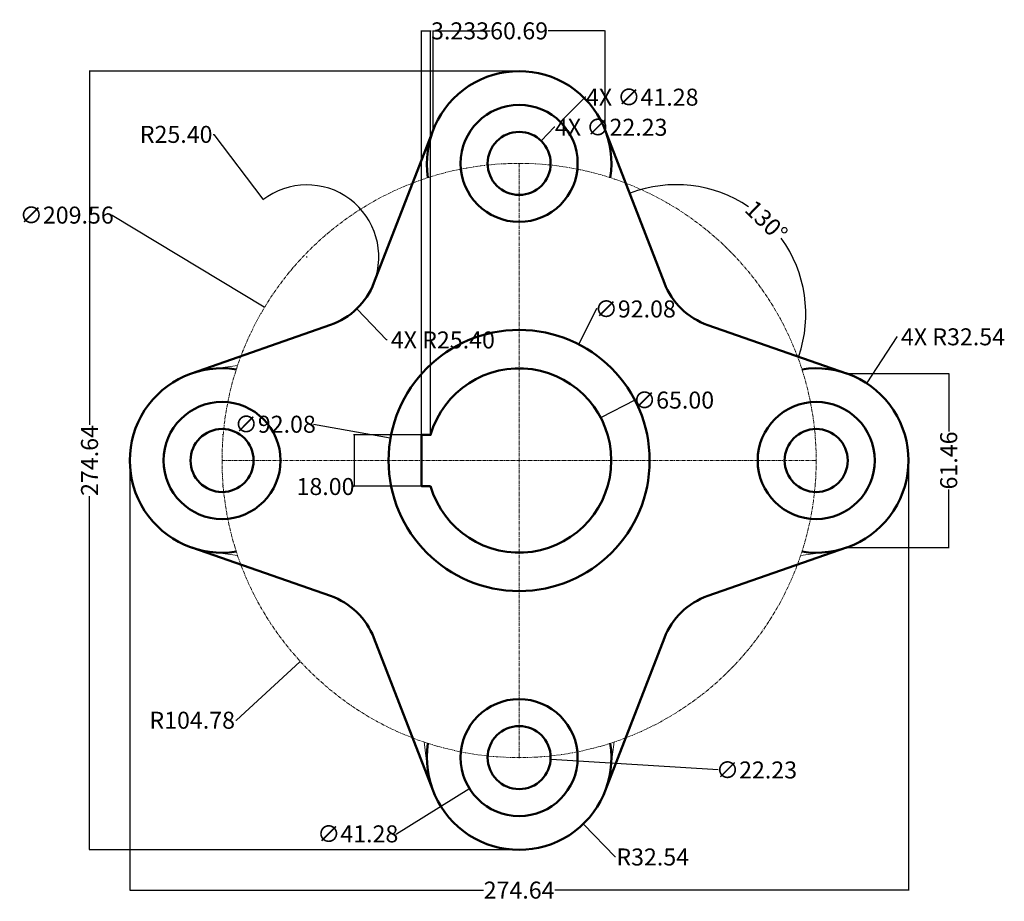
# Model space of a CAD drawing. Units: millimetres. Extents: x 95 to 442, y 57 to 368.
import ezdxf

# ---------------------------------------------------------------- set-up
doc = ezdxf.new("R2010")
doc.units = ezdxf.units.MM
doc.header["$MEASUREMENT"] = 0
doc.linetypes.add('CENTER', pattern=[2, 1.25, -0.25, 0.25, -0.25])
for name, color, linetype, lineweight in [('M-CNTR', 4, 'CENTER', 18), ('M-CONS', 8, 'Continuous', 13), ('M-DIMS', 2, 'Continuous', 25), ('M-OUTL', 7, 'Continuous', 50)]:
    doc.layers.add(name, color=color, linetype=linetype, lineweight=lineweight)
doc.styles.get("Standard").update_dxf_attribs({"font": 'arial.ttf'})
doc.dimstyles.get("Standard").update_dxf_attribs({"dimtxt": 6, "dimasz": 0.18, "dimexe": 0.18, "dimexo": 0.0625, "dimgap": 0.09, "dimtad": 0, "dimtoh": 1, "dimzin": 0, "dimdsep": 46, "dimtxsty": 'Standard', "dimcen": 0.09, "dimadec": 0, "dimazin": 0, "dimtfac": 1, "dimtofl": 0, "dimtmove": 0, "dimatfit": 3, "dimfxl": 1, "dimtolj": 1, "dimtzin": 0, "dimarcsym": 0})

# ---------------------------------------------------------------- blocks, each defined once
blk = doc.blocks.new('*D1')
at = {"layer": 'Defpoints', "color": 0, "transparency": 16777216}
for p in [(301.5, 329.2), (368.24, 283.05), (322.37, 275.25), (337.71, 260.43), (386.63, 243.41)]:
    blk.add_point(p, dxfattribs=at)
at = {"layer": 'M-DIMS', "color": 0, "lineweight": -2, "transparency": 16777216}
for start, end in [(56.1057, 110.9312), (341.0344, 35.8599)]:
    blk.add_arc((326.62, 264.3), 45.65, start, end, dxfattribs=at)
at = {"layer": 'M-DIMS', "color": 0, "transparency": 16777216}
for points in [[(310.32, 306.91), (310.3, 306.96), (310.14, 306.87)], [(369.82, 249.45), (369.76, 249.47), (369.73, 249.29)]]:
    blk.add_solid(points, dxfattribs=at)
at = {"layer": 'M-DIMS', "color": 0, "transparency": 16777216, "insert": (358.34, 297.13), "char_height": 6, "attachment_point": 5, "rotation": 315.9828}
blk.add_mtext('\\A1;130°', dxfattribs=at)
blk = doc.blocks.new('*D2')
at = {"layer": 'Defpoints', "color": 0, "transparency": 16777216}
for p in [(236.69, 221.68), (212.96, 203.68), (236.69, 203.68)]:
    blk.add_point(p, dxfattribs=at)
at = {"layer": 'M-DIMS', "color": 0, "lineweight": -2, "transparency": 16777216}
for p, q in [((236.63, 221.68), (212.78, 221.68)), ((212.96, 221.5), (212.96, 203.86)), ((236.63, 203.68), (212.78, 203.68)), ((212.96, 203.5), (212.78, 203.5)), ((212.96, 203.68), (212.96, 203.5))]:
    blk.add_line(p, q, dxfattribs=at)
at = {"layer": 'M-DIMS', "color": 0, "transparency": 16777216}
for points in [[(212.93, 221.5), (212.99, 221.5), (212.96, 221.68)], [(212.93, 203.86), (212.99, 203.86), (212.96, 203.68)]]:
    blk.add_solid(points, dxfattribs=at)
at = {"layer": 'M-DIMS', "color": 0, "transparency": 16777216, "insert": (202.86, 203.5), "char_height": 6, "attachment_point": 5}
blk.add_mtext('\\A1;18.00', dxfattribs=at)
blk = doc.blocks.new('*D3')
at = {"layer": 'Defpoints', "color": 0, "transparency": 16777216}
for p in [(299.96, 227.72), (242.34, 197.64)]:
    blk.add_point(p, dxfattribs=at)
at = {"layer": 'M-DIMS', "color": 0, "lineweight": -2, "transparency": 16777216}
for p, q in [((311.96, 233.98), (300.12, 227.8)), ((312.14, 233.98), (311.96, 233.98)), ((271.06, 212.68), (271.24, 212.68)), ((271.15, 212.59), (271.15, 212.77))]:
    blk.add_line(p, q, dxfattribs=at)
at = {"layer": 'M-DIMS', "color": 0, "transparency": 16777216}
blk.add_solid([(300.11, 227.83), (300.13, 227.77), (299.96, 227.72)], dxfattribs=at)
at = {"layer": 'M-DIMS', "color": 0, "transparency": 16777216, "insert": (325.61, 233.98), "char_height": 6, "attachment_point": 5}
blk.add_mtext('\\A1;∅65.00', dxfattribs=at)
blk = doc.blocks.new('*D4')
at = {"layer": 'Defpoints', "color": 0, "transparency": 16777216}
for p in [(292.09, 253.68), (250.21, 171.68)]:
    blk.add_point(p, dxfattribs=at)
at = {"layer": 'M-DIMS', "color": 0, "lineweight": -2, "transparency": 16777216}
for p, q in [((298.45, 266.12), (292.17, 253.84)), ((298.63, 266.12), (298.45, 266.12)), ((271.06, 212.68), (271.24, 212.68)), ((271.15, 212.59), (271.15, 212.77))]:
    blk.add_line(p, q, dxfattribs=at)
at = {"layer": 'M-DIMS', "color": 0, "transparency": 16777216}
blk.add_solid([(292.15, 253.85), (292.2, 253.82), (292.09, 253.68)], dxfattribs=at)
at = {"layer": 'M-DIMS', "color": 0, "transparency": 16777216, "insert": (312.11, 266.12), "char_height": 6, "attachment_point": 5}
blk.add_mtext('\\A1;∅92.08', dxfattribs=at)
blk = doc.blocks.new('*D5')
at = {"layer": 'Defpoints', "color": 0, "transparency": 16777216}
for p in [(180.89, 304.71), (196.26, 284.49)]:
    blk.add_point(p, dxfattribs=at)
at = {"layer": 'M-DIMS', "color": 0, "lineweight": -2, "transparency": 16777216}
for p, q in [((163.25, 327.69), (163.43, 327.69)), ((163.43, 327.69), (180.78, 304.85)), ((196.17, 284.49), (196.35, 284.49)), ((196.26, 284.4), (196.26, 284.58))]:
    blk.add_line(p, q, dxfattribs=at)
blk.add_arc((196.26, 284.49), 25.4, 338.9823, 127.6354, dxfattribs=at)
at = {"layer": 'M-DIMS', "color": 0, "transparency": 16777216}
blk.add_solid([(180.81, 304.87), (180.76, 304.84), (180.89, 304.71)], dxfattribs=at)
at = {"layer": 'M-DIMS', "color": 0, "transparency": 16777216, "insert": (150.18, 327.69), "char_height": 6, "attachment_point": 5}
blk.add_mtext('\\A1;R25.40', dxfattribs=at)
blk = doc.blocks.new('*D6')
at = {"layer": 'Defpoints', "color": 0, "transparency": 16777216}
for p in [(288.68, 118.79), (253.62, 97)]:
    blk.add_point(p, dxfattribs=at)
at = {"layer": 'M-DIMS', "color": 0, "lineweight": -2, "transparency": 16777216}
for p, q in [((271.06, 107.9), (271.24, 107.9)), ((271.15, 107.81), (271.15, 107.99)), ((227.88, 81), (253.47, 96.9)), ((227.7, 81), (227.88, 81))]:
    blk.add_line(p, q, dxfattribs=at)
at = {"layer": 'M-DIMS', "color": 0, "transparency": 16777216}
blk.add_solid([(253.45, 96.93), (253.48, 96.88), (253.62, 97)], dxfattribs=at)
at = {"layer": 'M-DIMS', "color": 0, "transparency": 16777216, "insert": (214.22, 81), "char_height": 6, "attachment_point": 5}
blk.add_mtext('\\A1;∅41.28', dxfattribs=at)
blk = doc.blocks.new('*D7')
at = {"layer": 'Defpoints', "color": 0, "transparency": 16777216}
for p in [(260.06, 108.58), (282.24, 107.21)]:
    blk.add_point(p, dxfattribs=at)
at = {"layer": 'M-DIMS', "color": 0, "lineweight": -2, "transparency": 16777216}
for p, q in [((271.06, 107.9), (271.24, 107.9)), ((271.15, 107.81), (271.15, 107.99)), ((341.4, 103.54), (282.42, 107.2))]:
    blk.add_line(p, q, dxfattribs=at)
at = {"layer": 'M-DIMS', "color": 0, "transparency": 16777216}
blk.add_solid([(282.43, 107.23), (282.42, 107.17), (282.24, 107.21)], dxfattribs=at)
at = {"layer": 'M-DIMS', "color": 0, "transparency": 16777216, "insert": (354.87, 103.54), "char_height": 6, "attachment_point": 5}
blk.add_mtext('\\A1;∅22.23', dxfattribs=at)
blk = doc.blocks.new('*D8')
at = {"layer": 'Defpoints', "color": 0, "transparency": 16777216}
for p in [(271.15, 107.9), (293.77, 84.5)]:
    blk.add_point(p, dxfattribs=at)
at = {"layer": 'M-DIMS', "color": 0, "lineweight": -2, "transparency": 16777216}
for p, q in [((271.06, 107.9), (271.24, 107.9)), ((271.15, 107.81), (271.15, 107.99)), ((305.02, 72.85), (293.89, 84.37)), ((305.2, 72.85), (305.02, 72.85))]:
    blk.add_line(p, q, dxfattribs=at)
at = {"layer": 'M-DIMS', "color": 0, "transparency": 16777216}
blk.add_solid([(293.91, 84.39), (293.87, 84.35), (293.77, 84.5)], dxfattribs=at)
at = {"layer": 'M-DIMS', "color": 0, "transparency": 16777216, "insert": (318.27, 72.85), "char_height": 6, "attachment_point": 5}
blk.add_mtext('\\A1;R32.54', dxfattribs=at)
blk = doc.blocks.new('*D9')
at = {"layer": 'Defpoints', "color": 0, "transparency": 16777216}
for p in [(271.15, 212.68), (193.99, 141.79)]:
    blk.add_point(p, dxfattribs=at)
at = {"layer": 'M-DIMS', "color": 0, "lineweight": -2, "transparency": 16777216}
for p, q in [((271.06, 212.68), (271.24, 212.68)), ((271.15, 212.59), (271.15, 212.77)), ((171.44, 121.08), (193.86, 141.67)), ((171.26, 121.08), (171.44, 121.08))]:
    blk.add_line(p, q, dxfattribs=at)
at = {"layer": 'M-DIMS', "color": 0, "transparency": 16777216}
blk.add_solid([(193.83, 141.69), (193.88, 141.65), (193.99, 141.79)], dxfattribs=at)
at = {"layer": 'M-DIMS', "color": 0, "transparency": 16777216, "insert": (155.84, 121.08), "char_height": 6, "attachment_point": 5}
blk.add_mtext('\\A1;R104.78', dxfattribs=at)
blk = doc.blocks.new('FLANGE-HOLE-22_23-CBORE-41_28')
for radius in [20.64, 11.12]:
    blk.add_circle((0, 0), radius)
blk = doc.blocks.new('*D11')
at = {"layer": 'Defpoints', "color": 0, "transparency": 16777216}
for p in [(119.63, 350), (271.15, 350), (271.15, 75.36)]:
    blk.add_point(p, dxfattribs=at)
at = {"layer": 'M-DIMS', "color": 0, "lineweight": -2, "transparency": 16777216}
for p, q in [((271.09, 350), (119.45, 350)), ((119.63, 349.82), (119.63, 225.26)), ((119.63, 75.54), (119.63, 200.09)), ((271.09, 75.36), (119.45, 75.36))]:
    blk.add_line(p, q, dxfattribs=at)
at = {"layer": 'M-DIMS', "color": 0, "transparency": 16777216}
for points in [[(119.6, 349.82), (119.66, 349.82), (119.63, 350)], [(119.6, 75.54), (119.66, 75.54), (119.63, 75.36)]]:
    blk.add_solid(points, dxfattribs=at)
at = {"layer": 'M-DIMS', "color": 0, "transparency": 16777216, "insert": (119.63, 212.68), "char_height": 6, "attachment_point": 5, "rotation": 90}
blk.add_mtext('\\A1;274.64', dxfattribs=at)
blk = doc.blocks.new('*D12')
at = {"layer": 'Defpoints', "color": 0, "transparency": 16777216}
for p in [(133.83, 212.68), (408.47, 212.68), (408.47, 61.16)]:
    blk.add_point(p, dxfattribs=at)
at = {"layer": 'M-DIMS', "color": 0, "lineweight": -2, "transparency": 16777216}
for p, q in [((133.83, 212.61), (133.83, 60.98)), ((408.47, 212.61), (408.47, 60.98)), ((134.01, 61.16), (258.57, 61.16)), ((408.29, 61.16), (283.73, 61.16))]:
    blk.add_line(p, q, dxfattribs=at)
at = {"layer": 'M-DIMS', "color": 0, "transparency": 16777216}
for points in [[(134.01, 61.19), (134.01, 61.13), (133.83, 61.16)], [(408.29, 61.19), (408.29, 61.13), (408.47, 61.16)]]:
    blk.add_solid(points, dxfattribs=at)
at = {"layer": 'M-DIMS', "color": 0, "transparency": 16777216, "insert": (271.15, 61.16), "char_height": 6, "attachment_point": 5}
blk.add_mtext('\\A1;274.64', dxfattribs=at)
blk = doc.blocks.new('*D13')
at = {"layer": 'Defpoints', "color": 0, "transparency": 16777216}
for p in [(301.5, 364.2), (240.8, 329.2), (301.5, 329.2)]:
    blk.add_point(p, dxfattribs=at)
at = {"layer": 'M-DIMS', "color": 0, "lineweight": -2, "transparency": 16777216}
for p, q in [((240.8, 329.26), (240.8, 364.38)), ((240.98, 364.2), (260.91, 364.2)), ((301.32, 364.2), (281.39, 364.2)), ((301.5, 329.26), (301.5, 364.38))]:
    blk.add_line(p, q, dxfattribs=at)
at = {"layer": 'M-DIMS', "color": 0, "transparency": 16777216}
for points in [[(240.98, 364.23), (240.98, 364.17), (240.8, 364.2)], [(301.32, 364.23), (301.32, 364.17), (301.5, 364.2)]]:
    blk.add_solid(points, dxfattribs=at)
at = {"layer": 'M-DIMS', "color": 0, "transparency": 16777216, "insert": (271.15, 364.2), "char_height": 6, "attachment_point": 5}
blk.add_mtext('\\A1;60.69', dxfattribs=at)
blk = doc.blocks.new('*D14')
at = {"layer": 'Defpoints', "color": 0, "transparency": 16777216}
for p in [(386.63, 243.41), (386.63, 181.95), (422.67, 181.95)]:
    blk.add_point(p, dxfattribs=at)
at = {"layer": 'M-DIMS', "color": 0, "lineweight": -2, "transparency": 16777216}
for p, q in [((386.69, 243.41), (422.85, 243.41)), ((422.67, 243.23), (422.67, 222.9)), ((422.67, 182.13), (422.67, 202.45)), ((386.69, 181.95), (422.85, 181.95))]:
    blk.add_line(p, q, dxfattribs=at)
at = {"layer": 'M-DIMS', "color": 0, "transparency": 16777216}
for points in [[(422.64, 243.23), (422.7, 243.23), (422.67, 243.41)], [(422.64, 182.13), (422.7, 182.13), (422.67, 181.95)]]:
    blk.add_solid(points, dxfattribs=at)
at = {"layer": 'M-DIMS', "color": 0, "transparency": 16777216, "insert": (422.67, 212.68), "char_height": 6, "attachment_point": 5, "rotation": 90}
blk.add_mtext('\\A1;61.46', dxfattribs=at)
blk = doc.blocks.new('*D15')
at = {"layer": 'Defpoints', "color": 0, "transparency": 16777216}
for p in [(239.92, 364.2), (236.69, 221.68), (239.92, 221.68)]:
    blk.add_point(p, dxfattribs=at)
at = {"layer": 'M-DIMS', "color": 0, "lineweight": -2, "transparency": 16777216}
for p, q in [((236.69, 221.74), (236.69, 364.38)), ((236.87, 364.2), (239.74, 364.2)), ((239.92, 221.74), (239.92, 364.38)), ((239.92, 364.2), (240.1, 364.2))]:
    blk.add_line(p, q, dxfattribs=at)
at = {"layer": 'M-DIMS', "color": 0, "transparency": 16777216}
for points in [[(236.87, 364.23), (236.87, 364.17), (236.69, 364.2)], [(239.74, 364.23), (239.74, 364.17), (239.92, 364.2)]]:
    blk.add_solid(points, dxfattribs=at)
at = {"layer": 'M-DIMS', "color": 0, "transparency": 16777216, "insert": (250.31, 364.2), "char_height": 6, "attachment_point": 5}
blk.add_mtext('\\A1;3.233', dxfattribs=at)
blk = doc.blocks.new('*D16')
at = {"layer": 'Defpoints', "color": 0, "transparency": 16777216}
for p in [(225.81, 220.67), (316.49, 204.68)]:
    blk.add_point(p, dxfattribs=at)
at = {"layer": 'M-DIMS', "color": 0, "lineweight": -2, "transparency": 16777216}
for p, q in [((198.6, 225.47), (225.63, 220.7)), ((271.06, 212.68), (271.24, 212.68)), ((271.15, 212.59), (271.15, 212.77))]:
    blk.add_line(p, q, dxfattribs=at)
at = {"layer": 'M-DIMS', "color": 0, "transparency": 16777216}
blk.add_solid([(225.64, 220.73), (225.63, 220.67), (225.81, 220.67)], dxfattribs=at)
at = {"layer": 'M-DIMS', "color": 0, "transparency": 16777216, "insert": (185.12, 225.47), "char_height": 6, "attachment_point": 5}
blk.add_mtext('\\A1;∅92.08', dxfattribs=at)
blk = doc.blocks.new('*D17')
at = {"layer": 'Defpoints', "color": 0, "transparency": 16777216}
for p in [(181.41, 266.77), (360.89, 158.58)]:
    blk.add_point(p, dxfattribs=at)
at = {"layer": 'M-DIMS', "color": 0, "lineweight": -2, "transparency": 16777216}
for p, q in [((127.39, 299.22), (127.57, 299.22)), ((127.57, 299.22), (181.26, 266.86)), ((271.06, 212.68), (271.24, 212.68)), ((271.15, 212.59), (271.15, 212.77))]:
    blk.add_line(p, q, dxfattribs=at)
at = {"layer": 'M-DIMS', "color": 0, "transparency": 16777216}
blk.add_solid([(181.27, 266.89), (181.24, 266.84), (181.41, 266.77)], dxfattribs=at)
at = {"layer": 'M-DIMS', "color": 0, "transparency": 16777216, "insert": (111.58, 299.22), "char_height": 6, "attachment_point": 5}
blk.add_mtext('\\A1;∅209.56', dxfattribs=at)
blk = doc.blocks.new('*D18')
at = {"layer": 'Defpoints', "color": 0, "transparency": 16777216}
for p in [(196.26, 284.49), (213.87, 266.18)]:
    blk.add_point(p, dxfattribs=at)
at = {"layer": 'M-DIMS', "color": 0, "lineweight": -2, "transparency": 16777216}
for p, q in [((196.17, 284.49), (196.35, 284.49)), ((196.26, 284.4), (196.26, 284.58)), ((224.43, 255.19), (213.99, 266.05)), ((224.61, 255.19), (224.43, 255.19))]:
    blk.add_line(p, q, dxfattribs=at)
at = {"layer": 'M-DIMS', "color": 0, "transparency": 16777216}
blk.add_solid([(214.01, 266.07), (213.97, 266.03), (213.87, 266.18)], dxfattribs=at)
at = {"layer": 'M-DIMS', "color": 0, "transparency": 16777216, "insert": (244.25, 255.19), "char_height": 6, "attachment_point": 5}
blk.add_mtext('\\A1;4X R25.40', dxfattribs=at)
blk = doc.blocks.new('*D19')
at = {"layer": 'Defpoints', "color": 0, "transparency": 16777216}
for p in [(393.7, 239.94), (375.93, 212.68)]:
    blk.add_point(p, dxfattribs=at)
at = {"layer": 'M-DIMS', "color": 0, "lineweight": -2, "transparency": 16777216}
for p, q in [((404.36, 256.29), (393.8, 240.09)), ((404.54, 256.29), (404.36, 256.29)), ((375.84, 212.68), (376.02, 212.68)), ((375.93, 212.59), (375.93, 212.77))]:
    blk.add_line(p, q, dxfattribs=at)
at = {"layer": 'M-DIMS', "color": 0, "transparency": 16777216}
blk.add_solid([(393.77, 240.1), (393.82, 240.07), (393.7, 239.94)], dxfattribs=at)
at = {"layer": 'M-DIMS', "color": 0, "transparency": 16777216, "insert": (424.18, 256.29), "char_height": 6, "attachment_point": 5}
blk.add_mtext('\\A1;4X R32.54', dxfattribs=at)
blk = doc.blocks.new('*D20')
at = {"layer": 'Defpoints', "color": 0, "transparency": 16777216}
for p in [(285.74, 332.05), (256.56, 302.86)]:
    blk.add_point(p, dxfattribs=at)
at = {"layer": 'M-DIMS', "color": 0, "lineweight": -2, "transparency": 16777216}
for p, q in [((294.5, 340.81), (285.87, 332.18)), ((294.68, 340.81), (294.5, 340.81)), ((271.06, 317.46), (271.24, 317.46)), ((271.15, 317.37), (271.15, 317.55))]:
    blk.add_line(p, q, dxfattribs=at)
at = {"layer": 'M-DIMS', "color": 0, "transparency": 16777216}
blk.add_solid([(285.85, 332.2), (285.89, 332.16), (285.74, 332.05)], dxfattribs=at)
at = {"layer": 'M-DIMS', "color": 0, "transparency": 16777216, "insert": (314.57, 340.81), "char_height": 6, "attachment_point": 5}
blk.add_mtext('\\A1;4X ∅41.28', dxfattribs=at)
blk = doc.blocks.new('*D21')
at = {"layer": 'Defpoints', "color": 0, "transparency": 16777216}
for p in [(278.9, 325.42), (263.4, 309.49)]:
    blk.add_point(p, dxfattribs=at)
at = {"layer": 'M-DIMS', "color": 0, "lineweight": -2, "transparency": 16777216}
for p, q in [((283.55, 330.2), (279.03, 325.55)), ((283.73, 330.2), (283.55, 330.2)), ((271.06, 317.46), (271.24, 317.46)), ((271.15, 317.37), (271.15, 317.55))]:
    blk.add_line(p, q, dxfattribs=at)
at = {"layer": 'M-DIMS', "color": 0, "transparency": 16777216}
blk.add_solid([(279.01, 325.57), (279.05, 325.53), (278.9, 325.42)], dxfattribs=at)
at = {"layer": 'M-DIMS', "color": 0, "transparency": 16777216, "insert": (303.62, 330.2), "char_height": 6, "attachment_point": 5}
blk.add_mtext('\\A1;4X ∅22.23', dxfattribs=at)

msp = doc.modelspace()

# ---------------------------------------------------------------- linework, layer by layer
at = {"layer": 'M-CNTR'}
for p, q in [((271.15, 317.4567), (271.15, 107.8967)), ((166.37, 221.6767), (166.7572, 221.6767)), ((166.37, 212.6767), (375.93, 212.6767)), ((166.37, 203.6767), (166.7572, 203.6767))]:
    msp.add_line(p, q, dxfattribs=at)
msp.add_circle((271.15, 212.6767), 104.78, dxfattribs=at)
at = {"layer": 'M-CONS'}
for p, q in [((303.69, 317.4567), (303.69, 317.4567)), ((162.1775, 244.9455), (171.8795, 246.206)), ((162.1775, 180.4079), (171.8795, 179.1474)), ((380.1225, 180.4079), (370.4205, 179.1474)), ((219.9484, 150.0391), (219.9484, 150.0367)), ((238.8812, 103.7042), (237.6207, 113.4062)), ((303.4188, 103.7042), (304.6793, 113.4062))]:
    msp.add_line(p, q, dxfattribs=at)
at = {"layer": 'M-OUTL'}
for points in [[(155.6417, 243.3973), (204.635, 260.5069, 0.21982273), (219.9484, 275.3185), (240.8037, 329.2021)], [(386.6268, 243.4083), (337.713, 260.4337, -0.22009924), (322.3748, 275.2546), (301.4966, 329.2013)], [(155.6733, 181.9451), (204.587, 164.9197, -0.22009924), (219.9252, 150.0988), (240.8034, 96.1521)], [(386.6268, 181.9451), (337.713, 164.9197, 0.22009924), (322.3748, 150.0988), (301.4966, 96.1521)]]:
    msp.add_lwpolyline(points, format="xyb", dxfattribs=at)
msp.add_lwpolyline([(239.921, 203.6767), (236.6882, 203.6767), (236.6882, 221.6767), (239.921, 221.6767, -7.08099922)], format="xyb", close=True, dxfattribs=at)
msp.add_circle((271.15, 212.6767), 46.04, dxfattribs=at)
for centre, start, end in [((271.15, 317.4567), 351.067096, 188.932904), ((166.37, 212.6767), 81.067096, 278.932904), ((375.93, 212.6767), 261.067096, 98.932904), ((271.15, 107.8967), 171.067096, 8.932904)]:
    msp.add_arc(centre, 32.54, start, end, dxfattribs=at)

# ---------------------------------------------------------------- block references
for p in [(271.15, 317.4567), (166.37, 212.6767), (375.93, 212.6767), (271.15, 107.8967)]:
    msp.add_blockref('FLANGE-HOLE-22_23-CBORE-41_28', p, dxfattribs=at)

# ---------------------------------------------------------------- dimensions: what is measured, and where the dimension line sits
at = {"layer": 'M-DIMS'}
for base, p1, p2, override, picture, middle in [((239.921, 364.1967), (236.6882, 221.6767), (239.921, 221.6767), {"dimdec": 3, "dimlfac": 1, "dimrnd": 0, "dimzin": 0, "dimdsep": 46, "dimlunit": 2}, '*D15', (250.3124, 364.1967)), ((301.4966, 364.1967), (240.8037, 329.2021), (301.4966, 329.2013), {"dimdec": 2, "dimlfac": 1, "dimrnd": 0, "dimzin": 0, "dimdsep": 46, "dimlunit": 2}, '*D13', (271.1502, 364.1967)), ((408.47, 61.1567), (133.83, 212.6767), (408.47, 212.6767), {"dimdec": 2, "dimlfac": 1, "dimrnd": 0, "dimzin": 0, "dimdsep": 46, "dimlunit": 2}, '*D12', (271.15, 61.1567))]:
    dim = msp.add_linear_dim(base=base, p1=p1, p2=p2, dimstyle='Standard', override=override, dxfattribs=at)
    dim.commit()
    dim.dimension.update_dxf_attribs({"geometry": picture, "text_midpoint": middle})
for base, p1, p2, override, picture, middle in [((119.63, 349.9967), (271.15, 75.3567), (271.15, 349.9967), {"dimdec": 2, "dimlfac": 1, "dimrnd": 0, "dimzin": 0, "dimdsep": 46, "dimlunit": 2}, '*D11', (119.63, 212.6767)), ((422.67, 181.9451), (386.6268, 243.4083), (386.6268, 181.9451), {"dimdec": 2, "dimlfac": 1, "dimrnd": 0, "dimzin": 0, "dimdsep": 46, "dimlunit": 2}, '*D14', (422.67, 212.6767)), ((212.9593, 203.6767), (236.6882, 221.6767), (236.6882, 203.6767), {"dimclrd": 0, "dimclre": 0, "dimclrt": 0}, '*D2', (202.8584, 203.4967))]:
    dim = msp.add_linear_dim(base=base, p1=p1, p2=p2, angle=90, dimstyle='Standard', override=override, dxfattribs=at)
    dim.commit()
    dim.dimension.update_dxf_attribs({"geometry": picture, "text_midpoint": middle})
for p1, p2, picture, middle in [((256.557, 302.8603), (285.743, 332.053), '*D20', (314.5697, 340.8108)), ((263.3979, 309.4912), (278.9021, 325.4221), '*D21', (303.618, 330.2014))]:
    dim = msp.add_diameter_dim_2p(p1=p1, p2=p2, text='4X <>', dimstyle='Standard', override={"dimdec": 2, "dimlfac": 1, "dimrnd": 0, "dimzin": 0, "dimdsep": 46, "dimlunit": 2}, dxfattribs=at)
    dim.commit()
    dim.dimension.update_dxf_attribs({"geometry": picture, "text_midpoint": middle, "dimtype": 163})
for center, mpoint, picture, middle in [((196.2607, 284.4867), (180.8935, 304.7107), '*D5', (150.1787, 327.6895)), ((271.15, 212.6767), (193.9877, 141.7907), '*D9', (155.8397, 121.0782)), ((271.15, 107.8967), (293.7654, 84.5002), '*D8', (318.2742, 72.8548))]:
    dim = msp.add_radius_dim(center=center, mpoint=mpoint, dimstyle='Standard', override={"dimclrd": 0, "dimclre": 0, "dimclrt": 0}, dxfattribs=at)
    dim.commit()
    dim.dimension.update_dxf_attribs({"geometry": picture, "text_midpoint": middle, "dimtype": 164})
dim = msp.add_angular_dim_2l(base=(368.237, 283.0524), line1=((386.6268, 243.4083), (337.713, 260.4337)), line2=((301.4966, 329.2013), (322.3748, 275.2546)), dimstyle='Standard', override={"dimclrd": 0, "dimclre": 0, "dimclrt": 0}, dxfattribs=at)
dim.commit()
dim.dimension.update_dxf_attribs({"geometry": '*D1', "text_midpoint": (358.3382, 297.1262)})
for p1, p2, override, picture, middle in [((360.8879, 158.5846), (181.4121, 266.7688), {"dimdec": 2, "dimlfac": 1, "dimrnd": 0, "dimzin": 0, "dimdsep": 46, "dimlunit": 2}, '*D17', (111.5831, 299.224)), ((250.2085, 171.675), (292.0915, 253.6783), {"dimclrd": 0, "dimclre": 0, "dimclrt": 0}, '*D4', (312.1093, 266.1193)), ((242.3401, 197.6354), (299.9599, 227.718), {"dimclrd": 0, "dimclre": 0, "dimclrt": 0}, '*D3', (325.6098, 233.9844)), ((316.4908, 204.6832), (225.8092, 220.6701), {"dimdec": 2, "dimlfac": 1, "dimrnd": 0, "dimzin": 0, "dimdsep": 46, "dimlunit": 2}, '*D16', (198.6048, 225.4662)), ((288.6783, 118.7947), (253.6217, 96.9986), {"dimclrd": 0, "dimclre": 0, "dimclrt": 0}, '*D6', (214.2202, 80.9964)), ((260.0563, 108.5843), (282.2437, 107.209), {"dimclrd": 0, "dimclre": 0, "dimclrt": 0}, '*D7', (341.3961, 103.5424))]:
    dim = msp.add_diameter_dim_2p(p1=p1, p2=p2, dimstyle='Standard', override=override, dxfattribs=at)
    dim.commit()
    dim.dimension.update_dxf_attribs({"geometry": picture, "text_midpoint": middle, "dimtype": 163})
for center, mpoint, picture, middle in [((196.2607, 284.4867), (213.866, 266.1778), '*D18', (244.2503, 255.1925)), ((375.93, 212.6767), (393.6982, 239.9373), '*D19', (424.1783, 256.2937))]:
    dim = msp.add_radius_dim(center=center, mpoint=mpoint, text='4X <>', dimstyle='Standard', override={"dimdec": 2, "dimlfac": 1, "dimrnd": 0, "dimzin": 0, "dimdsep": 46, "dimlunit": 2}, dxfattribs=at)
    dim.commit()
    dim.dimension.update_dxf_attribs({"geometry": picture, "text_midpoint": middle, "dimtype": 164})

doc.saveas('drawing.dxf')
